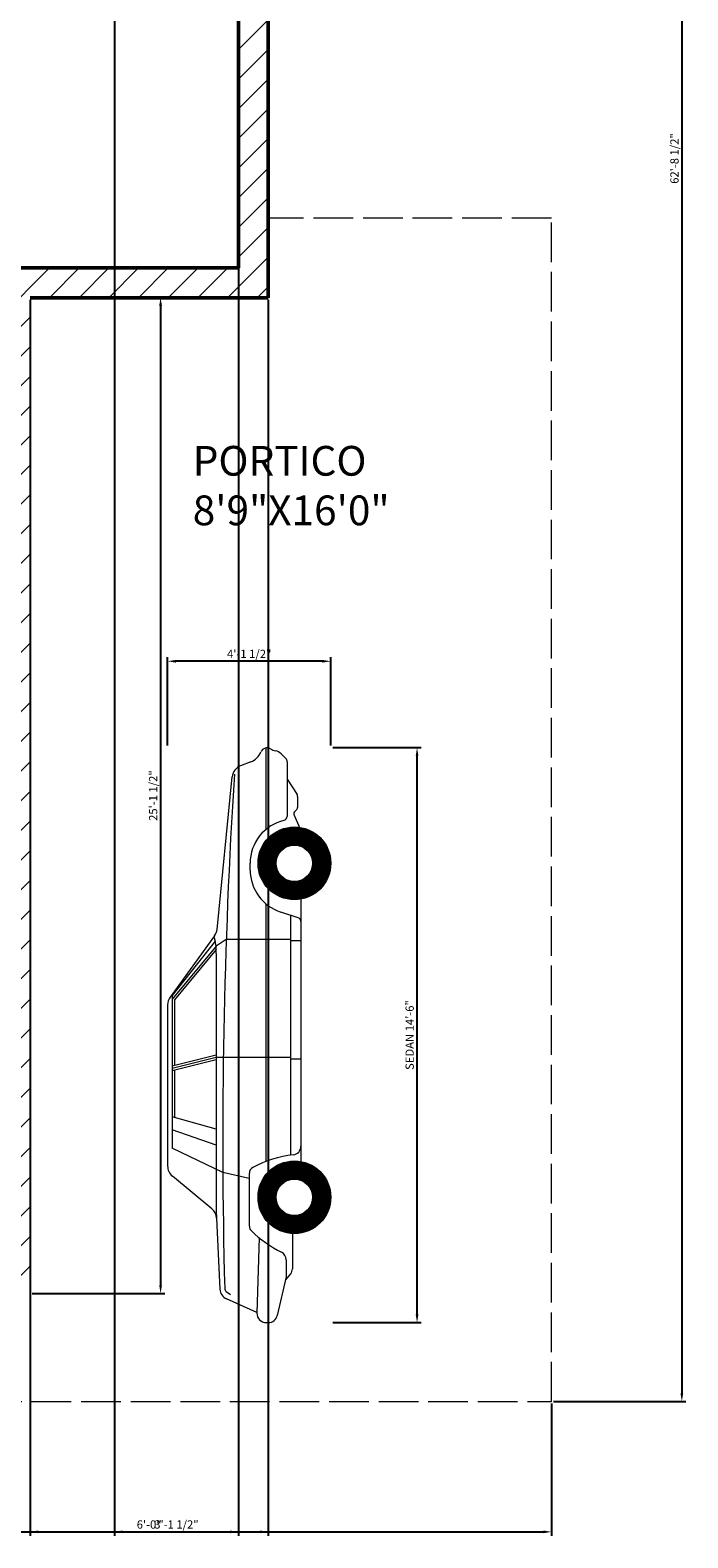
# Model space of a CAD drawing. Units: inches. Extents: x 2758 to 3288, y 1211 to 2050.
# Tile 2 of 4: x 3089 to 3288, y 1211 to 1667. Entities that reach past the tile are written whole.
import ezdxf

# ---------------------------------------------------------------- set-up
doc = ezdxf.new("R2010")
doc.units = ezdxf.units.IN
doc.linetypes.add('ACAD_ISO02W100', pattern=[15, 12, -3])
for name, color, linetype, lineweight in [('A-ANNO-DIMS', 2, 'Continuous', 18), ('A-AREA-IDEN', 7, 'Continuous', 25), ('A-EQPM-VEHI', 8, 'Continuous', 18), ('A-WALL', 7, 'Continuous', 50)]:
    doc.layers.add(name, color=color, linetype=linetype, lineweight=lineweight)
doc.layers.add('A-FLOR-OVHD', color=244, linetype='ACAD_ISO02W100', lineweight=18, true_color=0x991b1e)
doc.layers.add('A-WALL-PATT', color=244, linetype='Continuous', lineweight=13, true_color=0x991b1e)
doc.styles.get("Standard").update_dxf_attribs({"font": 'arial.ttf'})
doc.dimstyles.new('ISO-25', dxfattribs={"dimtxt": 2.5, "dimasz": 2.5, "dimexe": 1.25, "dimexo": 0.625, "dimtad": 1, "dimlunit": 3, "dimtxsty": 'Standard', "dimcen": 2.5, "dimadec": 0, "dimazin": 0, "dimtfac": 1, "dimtmove": 0, "dimatfit": 3, "dimfxl": 1, "dimarcsym": 0})

# ---------------------------------------------------------------- blocks, each defined once
blk = doc.blocks.new('Car - sedan  side')
for p, q in [((-139.53, 35.99), (-129.64, 47.91)), ((-128.57, 32.64), (-121.22, 48.02)), ((-77.81, 49.34), (-126.58, 49.34)), ((-74.7, 48.02), (-121.22, 48.02)), ((-120.32, 34.67), (-115.67, 48.02)), ((-115.4, 34.67), (-111.74, 48.02)), ((-97.55, 47.3), (-111.94, 47.3)), ((-94.41, 34.67), (-97.73, 48.02)), ((-93.72, 34.67), (-97.04, 48.02)), ((-93.03, 34.67), (-96.34, 48.02)), ((-76.26, 47.3), (-96.16, 47.3)), ((-61.08, 34.66), (-76.26, 47.3)), ((-60.02, 34.65), (-76.07, 48.02)), ((-56.87, 35.13), (-75.48, 48.59)), ((-58.54, 34.93), (-74.99, 48.02)), ((-140.23, 34.67), (-163.88, 33.56)), ((-62.28, 34.67), (-140.23, 34.67)), ((-130.39, 24.63), (-128.57, 32.64)), ((-93.72, 19.62), (-93.72, 34.67)), ((-62.28, 34.67), (-60.02, 34.65)), ((-60.02, 34.65), (-58.54, 34.93)), ((-57.97, 31.61), (-60.02, 34.65)), ((-57.21, 35.38), (-58.54, 34.93)), ((-54.93, 34.4), (-8.75, 29.8)), ((-170.93, 22.32), (-166.81, 31.56)), ((-164.57, 31.6), (-165.48, 30.35)), ((-57.97, 19.62), (-57.97, 31.61)), ((-128.78, 24.63), (-144.79, 24.63)), ((-36.97, 24.38), (-34.94, 24.38)), ((-4.21, 24.18), (-5.42, 27.27)), ((-174, 19.51), (-174, 18.91)), ((-148.26, 21.7), (-171.11, 22.33)), ((-47.2, 19.62), (-125.23, 19.62)), ((-93.72, 12.14), (-93.72, 19.62)), ((-57.97, 12.14), (-57.97, 19.62)), ((0, 19.62), (-24.7, 19.62)), ((-160.12, 13.48), (-171.81, 16.16)), ((-159.22, 12.14), (-161.08, 13.7)), ((-51.4, 9.89), (-49.69, 15.14)), ((-3.22, 13.59), (-1.77, 14.97)), ((-155.01, 13.48), (-160.12, 13.48)), ((-147.03, 11.6), (-157.73, 11.6)), ((-50.67, 12.14), (-123.32, 12.14)), ((-94.21, 9.03), (-94.21, 12.14)), ((-58.39, 9.03), (-58.39, 12.14)), ((-20.36, 11.06), (-24.06, 9.44)), ((-4.23, 13.19), (-20.72, 13.19)), ((-18.83, 10.42), (-19.11, 10.76)), ((-14.68, 10.03), (-18.01, 10.03)), ((-9.5, 13.19), (-14.1, 10.2)), ((-120.62, 9.03), (-125.23, 9.03)), ((-45.76, 9.03), (-120.62, 9.03))]:
    blk.add_line(p, q)
at = {"const_width": 5.49}
for points in [[(-127.8, 11, -1), (-144.3, 11, -1)], [(-26.69, 11, -1), (-43.19, 11, -1)]]:
    blk.add_lwpolyline(points, format="xyb", close=True, dxfattribs=at)
for centre, radius in [((-136.05, 11), 11), ((-34.94, 11), 11), ((-136.05, 11), 5.51), ((-34.94, 11), 5.51)]:
    blk.add_circle(centre, radius)
for centre, radius, start, end in [((-126.58, 45.38), 3.97, 90, 140.3029), ((-77.81, 45.38), 3.97, 54.135, 90), ((-163.72, 30.18), 3.38, 92.6827, 155.9736), ((-163.62, 30.91), 1.17, 91.491, 143.9553), ((-118.51, -1702.12), 1734.79, 86.34698, 91.49105), ((-142.58, 38.53), 3.97, 272.6827, 320.3029), ((-54.54, 38.35), 3.97, 234.135, 264.3123), ((-9.15, 25.82), 4, 21.3107, 84.3123), ((-118.09, -2.78), 38.85, 136.3964, 152.9097), ((-144.79, 22.64), 1.98, 90, 136.3964), ((-128.78, 22.64), 1.98, 28.1371, 90), ((-157.14, 7.48), 34.14, 6.5135, 28.1371), ((-36.97, 11), 13.38, 90, 161.9732), ((-34.94, 11), 13.38, 13.5864, 90), ((0.9, 26.18), 5.49, 201.3107, 247.7048), ((-171.18, 19.51), 2.82, 88.4193, 180), ((-171.18, 18.91), 2.82, 180, 257.0905), ((-1.92, 19.3), 1.94, 325.3744, 67.7048), ((-155.01, 16.1), 2.62, 270, 332.9097), ((-20.72, 14.43), 1.24, 193.5864, 270), ((-3.82, 17.12), 2.96, 313.7173, 352.3839), ((2.46, 16.28), 3.37, 145.3744, 172.3839), ((-157.73, 13.93), 2.32, 230.1291, 270), ((-120.62, 11.65), 2.62, 186.5135, 270), ((-52.58, 10.27), 1.24, 270, 341.9732), ((-19.93, 10.09), 1.06, 39.301, 113.7159), ((-18.01, 11.09), 1.06, 219.301, 270), ((-14.68, 11.09), 1.06, 270, 303.047), ((-4.23, 14.65), 1.46, 270, 313.7173)]:
    blk.add_arc(centre, radius, start, end)
blk = doc.blocks.new('*D14')
at = {"layer": 'A-ANNO-DIMS', "color": 0, "lineweight": -2, "transparency": 16777216}
for p, q in [((3180.69, 1450.11), (3207.43, 1450.11)), ((3206.18, 1278.5), (3206.18, 1447.61)), ((3180.69, 1276), (3207.43, 1276))]:
    blk.add_line(p, q, dxfattribs=at)
at = {"layer": 'A-ANNO-DIMS', "color": 0, "transparency": 16777216}
for points in [[(3205.77, 1447.61), (3206.6, 1447.61), (3206.18, 1450.11)], [(3205.77, 1278.5), (3206.6, 1278.5), (3206.18, 1276)]]:
    blk.add_solid(points, dxfattribs=at)
at = {"layer": 'Defpoints', "color": 0, "transparency": 16777216}
for p in [(3180.07, 1450.11), (3206.18, 1450.11), (3180.07, 1276)]:
    blk.add_point(p, dxfattribs=at)
at = {"layer": 'A-ANNO-DIMS', "color": 0, "transparency": 16777216, "insert": (3204.27, 1363.06), "char_height": 2.5, "attachment_point": 5, "rotation": 90}
blk.add_mtext('SEDAN 14\'-6"', dxfattribs=at)
blk = doc.blocks.new('*D15')
at = {"layer": 'A-ANNO-DIMS', "color": 0, "lineweight": -2, "transparency": 16777216}
for p, q in [((3130.72, 1450.74), (3130.72, 1477.48)), ((3177.57, 1476.23), (3133.22, 1476.23)), ((3180.07, 1450.74), (3180.07, 1477.48))]:
    blk.add_line(p, q, dxfattribs=at)
at = {"layer": 'A-ANNO-DIMS', "color": 0, "transparency": 16777216}
for points in [[(3133.22, 1476.65), (3133.22, 1475.82), (3130.72, 1476.23)], [(3177.57, 1476.65), (3177.57, 1475.82), (3180.07, 1476.23)]]:
    blk.add_solid(points, dxfattribs=at)
at = {"layer": 'Defpoints', "color": 0, "transparency": 16777216}
for p in [(3130.72, 1476.23), (3130.72, 1450.11), (3180.07, 1450.11)]:
    blk.add_point(p, dxfattribs=at)
at = {"layer": 'A-ANNO-DIMS', "color": 0, "transparency": 16777216, "insert": (3155.4, 1478.15), "char_height": 2.5, "attachment_point": 5}
blk.add_mtext('4\'-1 1/2"', dxfattribs=at)
blk = doc.blocks.new('*D18')
at = {"layer": 'A-ANNO-DIMS', "color": 0, "lineweight": -2, "transparency": 16777216}
for p, q in [((2801.14, 1284.19), (2801.14, 1211.4)), ((3246.84, 1251.47), (3246.84, 1211.4)), ((2803.64, 1212.65), (3244.34, 1212.65))]:
    blk.add_line(p, q, dxfattribs=at)
at = {"layer": 'A-ANNO-DIMS', "color": 0, "transparency": 16777216}
for points in [[(2803.64, 1213.06), (2803.64, 1212.23), (2801.14, 1212.65)], [(3244.34, 1213.06), (3244.34, 1212.23), (3246.84, 1212.65)]]:
    blk.add_solid(points, dxfattribs=at)
at = {"layer": 'Defpoints', "color": 0, "transparency": 16777216}
for p in [(2801.14, 1284.81), (3246.84, 1252.1), (3246.84, 1212.65)]:
    blk.add_point(p, dxfattribs=at)
at = {"layer": 'A-ANNO-DIMS', "color": 0, "transparency": 16777216, "insert": (3023.99, 1214.57), "char_height": 2.5, "attachment_point": 5}
blk.add_mtext('37\'-1 1/2"', dxfattribs=at)
blk = doc.blocks.new('*D19')
at = {"layer": 'A-ANNO-DIMS', "color": 0, "lineweight": -2, "transparency": 16777216}
for p, q in [((3161.76, 2004.81), (3287.54, 2004.81)), ((3286.29, 2002.31), (3286.29, 1254.6)), ((3247.46, 1252.1), (3287.54, 1252.1))]:
    blk.add_line(p, q, dxfattribs=at)
at = {"layer": 'A-ANNO-DIMS', "color": 0, "transparency": 16777216}
for points in [[(3285.87, 2002.31), (3286.7, 2002.31), (3286.29, 2004.81)], [(3285.87, 1254.6), (3286.7, 1254.6), (3286.29, 1252.1)]]:
    blk.add_solid(points, dxfattribs=at)
at = {"layer": 'Defpoints', "color": 0, "transparency": 16777216}
for p in [(3161.14, 2004.81), (3246.84, 1252.1), (3286.29, 1252.1)]:
    blk.add_point(p, dxfattribs=at)
at = {"layer": 'A-ANNO-DIMS', "color": 0, "transparency": 16777216, "insert": (3284.37, 1628.45), "char_height": 2.5, "attachment_point": 5, "rotation": 90}
blk.add_mtext('62\'-8 1/2"', dxfattribs=at)
blk = doc.blocks.new('*D20')
at = {"layer": 'A-ANNO-DIMS', "color": 0, "lineweight": -2, "transparency": 16777216}
for p, q in [((3089.14, 1585.69), (3089.14, 1211.4)), ((3161.14, 1585.69), (3161.14, 1211.4)), ((3091.64, 1212.65), (3158.64, 1212.65))]:
    blk.add_line(p, q, dxfattribs=at)
at = {"layer": 'A-ANNO-DIMS', "color": 0, "transparency": 16777216}
for points in [[(3091.64, 1213.06), (3091.64, 1212.23), (3089.14, 1212.65)], [(3158.64, 1213.06), (3158.64, 1212.23), (3161.14, 1212.65)]]:
    blk.add_solid(points, dxfattribs=at)
at = {"layer": 'Defpoints', "color": 0, "transparency": 16777216}
for p in [(3089.14, 1586.31), (3161.14, 1586.31), (3161.14, 1212.65)]:
    blk.add_point(p, dxfattribs=at)
at = {"layer": 'A-ANNO-DIMS', "color": 0, "transparency": 16777216, "insert": (3125.14, 1214.55), "char_height": 2.5, "attachment_point": 5}
blk.add_mtext('6\'-0"', dxfattribs=at)
blk = doc.blocks.new('*D21')
at = {"layer": 'A-ANNO-DIMS', "color": 0, "lineweight": -2, "transparency": 16777216}
for p, q in [((3089.76, 1586.31), (3129.84, 1586.31)), ((3128.59, 1583.81), (3128.59, 1287.31)), ((3089.76, 1284.81), (3129.84, 1284.81))]:
    blk.add_line(p, q, dxfattribs=at)
at = {"layer": 'A-ANNO-DIMS', "color": 0, "transparency": 16777216}
for points in [[(3128.17, 1583.81), (3129.01, 1583.81), (3128.59, 1586.31)], [(3128.17, 1287.31), (3129.01, 1287.31), (3128.59, 1284.81)]]:
    blk.add_solid(points, dxfattribs=at)
at = {"layer": 'Defpoints', "color": 0, "transparency": 16777216}
for p in [(3089.14, 1586.31), (3089.14, 1284.81), (3128.59, 1284.81)]:
    blk.add_point(p, dxfattribs=at)
at = {"layer": 'A-ANNO-DIMS', "color": 0, "transparency": 16777216, "insert": (3126.67, 1435.56), "char_height": 2.5, "attachment_point": 5, "rotation": 90}
blk.add_mtext('25\'-1 1/2"', dxfattribs=at)
blk = doc.blocks.new('*D25')
at = {"layer": 'A-ANNO-DIMS', "color": 0, "lineweight": -2, "transparency": 16777216}
for p, q in [((3152.14, 1995.19), (3152.14, 1211.4)), ((3114.64, 1887.19), (3114.64, 1211.4)), ((3117.14, 1212.65), (3149.64, 1212.65))]:
    blk.add_line(p, q, dxfattribs=at)
at = {"layer": 'A-ANNO-DIMS', "color": 0, "transparency": 16777216}
for points in [[(3117.14, 1213.06), (3117.14, 1212.23), (3114.64, 1212.65)], [(3149.64, 1213.06), (3149.64, 1212.23), (3152.14, 1212.65)]]:
    blk.add_solid(points, dxfattribs=at)
at = {"layer": 'Defpoints', "color": 0, "transparency": 16777216}
for p in [(3152.14, 1995.81), (3114.64, 1887.81), (3152.14, 1212.65)]:
    blk.add_point(p, dxfattribs=at)
at = {"layer": 'A-ANNO-DIMS', "color": 0, "transparency": 16777216, "insert": (3133.39, 1214.57), "char_height": 2.5, "attachment_point": 5}
blk.add_mtext('3\'-1 1/2"', dxfattribs=at)

msp = doc.modelspace()

# ---------------------------------------------------------------- hatches: boundary and pattern name
at = {"layer": 'A-WALL-PATT'}
h = msp.add_hatch(dxfattribs=at)
h.set_pattern_fill('ANSI31', color=256, scale=2)
h.paths.add_polyline_path([(2810.139, 1377.81), (2810.139, 1715.31), (2939.691, 1715.31), (2939.691, 1724.31), (2910.639, 1724.31), (2910.639, 1778.31), (2906.139, 1778.31), (2906.139, 1724.31), (2896.389, 1724.31), (2810.139, 1724.31), (2810.139, 1796.31), (2982.639, 1796.31), (2982.639, 1800.81), (2810.139, 1800.81), (2810.139, 1920.81), (2872.139, 1920.81), (2872.139, 1929.81), (2810.139, 1929.81), (2810.139, 1995.81), (2890.139, 1995.81), (2890.139, 1920.81), (2973.639, 1920.81), (2973.639, 1841.31), (2949.639, 1841.31), (2949.639, 1836.81), (2973.639, 1836.81), (3114.639, 1836.81), (3114.639, 1887.81), (3110.139, 1887.81), (3110.139, 1845.81), (2982.639, 1845.81), (2982.639, 1977.81), (2973.639, 1977.81), (2973.639, 1929.81), (2894.639, 1929.81), (2894.639, 1995.81), (3152.139, 1995.81), (3152.139, 1800.81), (3152.139, 1796.31), (3152.139, 1724.31), (3074.139, 1724.31), (3074.139, 1715.31), (3152.139, 1715.31), (3152.139, 1595.31), (3020.139, 1595.31), (3020.139, 1667.31), (3011.139, 1667.31), (3011.139, 1586.31), (3080.139, 1586.31), (3080.139, 1284.81), (3089.139, 1284.81), (3089.139, 1586.31), (3161.139, 1586.31), (3161.139, 2004.81), (2801.139, 2004.81), (2801.139, 1284.81), (3032.139, 1284.81), (3032.139, 1320.81), (3023.139, 1320.81), (3023.139, 1293.81), (2810.139, 1293.81), (2810.139, 1368.81), (3032.139, 1368.81), (3032.139, 1377.81)])

# ---------------------------------------------------------------- linework, layer by layer
at = {"layer": 'A-FLOR-OVHD'}
for p, q in [((3246.836, 1610.37), (3161.139, 1610.37)), ((3246.836, 1252.097), (3246.836, 1610.37)), ((3014.57, 1252.097), (3246.836, 1252.097))]:
    msp.add_line(p, q, dxfattribs=at)
at = {"layer": 'A-WALL'}
for p, q in [((3161.139, 2004.81), (3161.139, 1586.31)), ((3152.139, 1715.31), (3152.139, 1595.31)), ((3020.139, 1595.31), (3152.139, 1595.31)), ((3089.139, 1586.31), (3161.139, 1586.31))]:
    msp.add_line(p, q, dxfattribs=at)

# ---------------------------------------------------------------- block references
at = {"layer": 'A-EQPM-VEHI', "rotation": 90}
msp.add_blockref('Car - sedan  side', (3180.068, 1450.001), dxfattribs=at)

# ---------------------------------------------------------------- texts
at = {"layer": 'A-AREA-IDEN', "insert": (3135.564, 1541.425), "char_height": 9, "attachment_point": 1}
msp.add_mtext_dynamic_manual_height_columns(' PORTICO\\P 8\'9"X16\'0"', width=130.32194, gutter_width=12.5, heights=[77.844], dxfattribs=at)

# ---------------------------------------------------------------- dimensions: what is measured, and where the dimension line sits
at = {"layer": 'A-ANNO-DIMS'}
for base, p1, p2, angle, picture, middle in [((3286.286, 1252.097), (3161.139, 2004.81), (3246.836, 1252.097), 90, '*D19', (3284.368, 1628.454)), ((3128.589, 1284.81), (3089.139, 1586.31), (3089.139, 1284.81), 270, '*D21', (3126.671, 1435.56)), ((3130.723, 1476.232), (3180.068, 1450.115), (3130.723, 1450.115), 180, '*D15', (3155.395, 1478.149))]:
    dim = msp.add_linear_dim(base=base, p1=p1, p2=p2, angle=angle, dimstyle='ISO-25', override={"dimdec": 1, "dimlfac": 1, "dimrnd": 0, "dimzin": 1, "dimdsep": 46, "dimlunit": 4, "dimfrac": 2}, dxfattribs=at)
    dim.commit()
    dim.dimension.update_dxf_attribs({"geometry": picture, "text_midpoint": middle})
for base, p1, p2, picture, middle in [((3152.139, 1212.647), (3114.639, 1887.81), (3152.139, 1995.81), '*D25', (3133.389, 1214.566)), ((3161.139, 1212.647), (3089.139, 1586.31), (3161.139, 1586.31), '*D20', (3125.139, 1214.549)), ((3246.836, 1212.647), (2801.139, 1284.81), (3246.836, 1252.097), '*D18', (3023.987, 1214.566))]:
    dim = msp.add_linear_dim(base=base, p1=p1, p2=p2, dimstyle='ISO-25', override={"dimdec": 1, "dimlfac": 1, "dimrnd": 0, "dimzin": 1, "dimdsep": 46, "dimlunit": 4, "dimfrac": 2}, dxfattribs=at)
    dim.commit()
    dim.dimension.update_dxf_attribs({"geometry": picture, "text_midpoint": middle})
dim = msp.add_linear_dim(base=(3206.185, 1450.115), p1=(3180.068, 1276.001), p2=(3180.068, 1450.115), angle=90, text='SEDAN <>', dimstyle='ISO-25', override={"dimdec": 1, "dimlfac": 1, "dimrnd": 0, "dimzin": 1, "dimdsep": 46, "dimlunit": 4, "dimfrac": 2}, dxfattribs=at)
dim.commit()
dim.dimension.update_dxf_attribs({"geometry": '*D14', "text_midpoint": (3204.267, 1363.058)})

doc.saveas('drawing.dxf')
